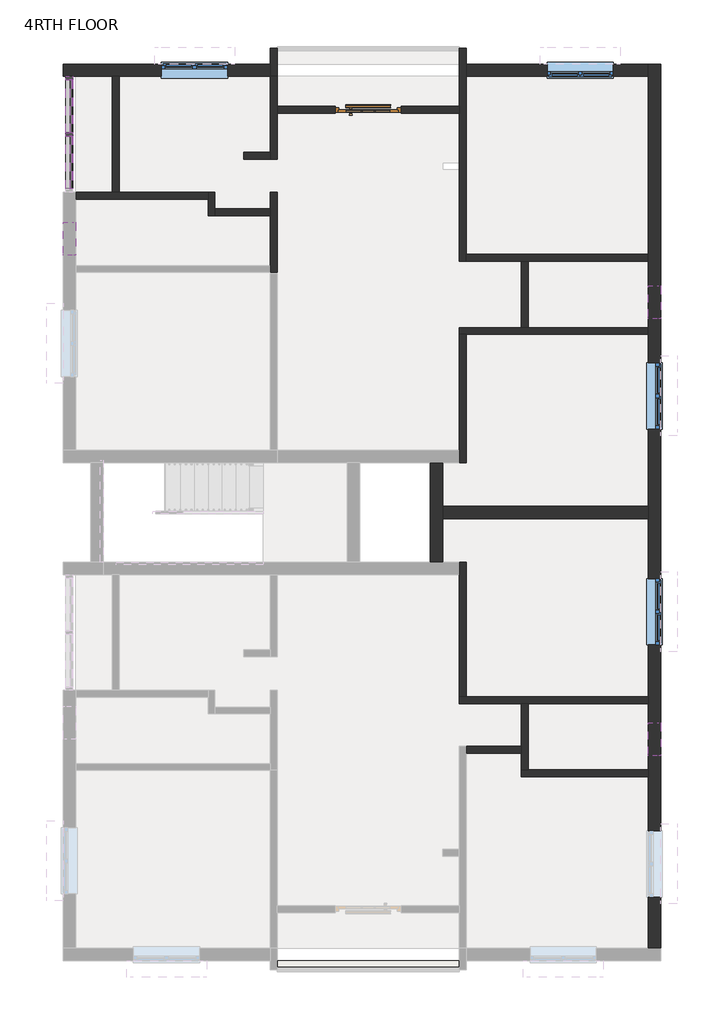
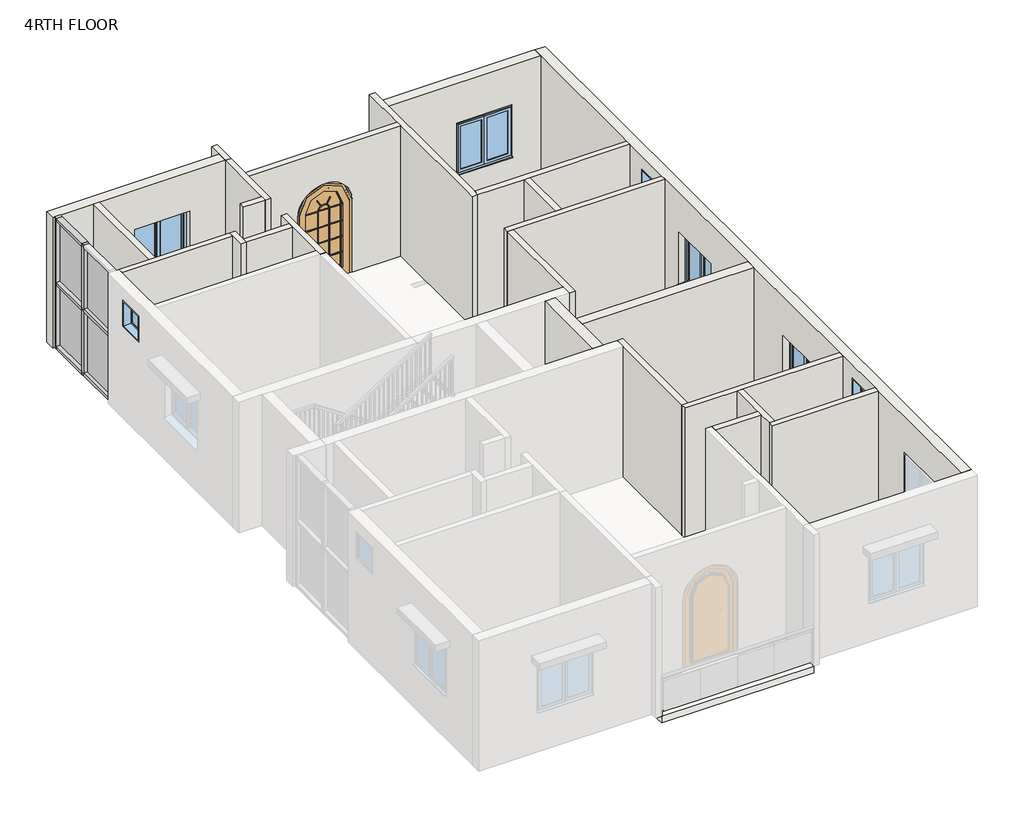
# One storey, part 2 of 4: 24 walls, 9 members, 7 windows, 4 plates, 1 door, 1 slab.
"""IFC4 building model written with IfcOpenShell, lengths in millimetres."""

from ifc_helpers import new_model, si_unit, point, frame, frame_2d, origin, place, context, project, spatial, polyline, circle_curve, trimmed, segment, composite_curve, outline, extrude, faceted_brep, transform, mapped, element, save
from components import door_arched_single_french_glass_wood_exterior_4_x_7_french_5c4dec95, member_801a2072, member_82905deb, member_88aa5c81, member_4491d118, system_panel_glazed_a8655be6, window_80340324, w2_windows_4_x_4_9dec5fc7

model = new_model("IFC4")

# Units and contexts
model_context = context("Model", 3, world=origin())
ifc_project = project(units=[si_unit("LENGTHUNIT", "METRE", prefix="MILLI")], contexts=[model_context])

# Site, building, storey
site = spatial("IfcSite", under=ifc_project)
building = spatial("IfcBuilding", under=site)
storey = spatial("IfcBuildingStorey", under=building, Name="4RTH FLOOR", Elevation=15240.0)

# Door
placement = place(None, origin())
door_arched_single_french_glass_wood_exterior_4_x_7_french_shape = door_arched_single_french_glass_wood_exterior_4_x_7_french_5c4dec95(model_context)
element("IfcDoor", 1, ObjectType="Door_Arched_Single_French_Glass_Wood_Exterior : 4' x 7' french door", at=placement, inside=storey, context=model_context, shape_type="MappedRepresentation", body=[
    mapped(door_arched_single_french_glass_wood_exterior_4_x_7_french_shape, transform((-817.6012202, 12433.0309003, 15240.0), x_axis=(1.0, 0.0, 0.0), y_axis=(0.0, 1.0, 0.0), z_axis=(0.0, 0.0, 1.0))),
])

# Members
member_shape = member_801a2072(model_context)
element("IfcMember", 2, ObjectType="Rectangular Mullion : 2.5\" x 5\" rectangular", at=placement, inside=storey, context=model_context, shape_type="MappedRepresentation", body=[
    mapped(member_shape, transform((-6318.2887202, 12007.5809003, 18288.0), x_axis=(0.0, 0.0, 1.0), y_axis=(-1.0, 0.0, 0.0), z_axis=(0.0, -1.0, 0.0))),
])
element("IfcMember", 3, ObjectType="Rectangular Mullion : 2.5\" x 5\" rectangular", at=placement, inside=storey, context=model_context, shape_type="MappedRepresentation", body=[
    mapped(member_shape, transform((-6318.2887202, 12979.1309003, 15240.0), x_axis=(0.0, 0.0, -1.0), y_axis=(-1.0, 0.0, 0.0), z_axis=(0.0, 1.0, 0.0))),
])
element("IfcMember", 4, ObjectType="Rectangular Mullion : 2.5\" x 5\" rectangular", at=placement, inside=storey, context=model_context, shape_type="MappedRepresentation", body=[
    mapped(member_shape, transform((-6318.2887202, 11944.0809003, 15240.0), x_axis=(0.0, 0.0, -1.0), y_axis=(-1.0, 0.0, 0.0), z_axis=(0.0, 1.0, 0.0))),
])
member_2_shape = member_82905deb(model_context)
element("IfcMember", 5, ObjectType="Rectangular Mullion : 2.5\" x 5\" rectangular", at=placement, inside=storey, context=model_context, shape_type="MappedRepresentation", body=[
    mapped(member_2_shape, transform((-6318.2887202, 11975.8309003, 15240.0), x_axis=(0.0, -1.0, 0.0), y_axis=(-1.0, 0.0, 0.0), z_axis=(0.0, 0.0, -1.0))),
])
member_3_shape = member_88aa5c81(model_context)
element("IfcMember", 6, ObjectType="Rectangular Mullion : 2.5\" x 5\" rectangular", at=placement, inside=storey, context=model_context, shape_type="MappedRepresentation", body=[
    mapped(member_3_shape, transform((-6318.2887202, 12007.5809003, 16764.0), x_axis=(0.0, 0.0, 1.0), y_axis=(-1.0, 0.0, 0.0), z_axis=(0.0, -1.0, 0.0))),
])
element("IfcMember", 7, ObjectType="Rectangular Mullion : 2.5\" x 5\" rectangular", at=placement, inside=storey, context=model_context, shape_type="MappedRepresentation", body=[
    mapped(member_3_shape, transform((-6318.2887202, 10972.5309003, 16764.0), x_axis=(0.0, 0.0, 1.0), y_axis=(-1.0, 0.0, 0.0), z_axis=(0.0, -1.0, 0.0))),
])
element("IfcMember", 8, ObjectType="Rectangular Mullion : 2.5\" x 5\" rectangular", at=placement, inside=storey, context=model_context, shape_type="MappedRepresentation", body=[
    mapped(member_2_shape, transform((-6318.2887202, 11975.8309003, 16764.0), x_axis=(0.0, -1.0, 0.0), y_axis=(-1.0, 0.0, 0.0), z_axis=(0.0, 0.0, -1.0))),
])
member_4_shape = member_4491d118(model_context)
element("IfcMember", 9, ObjectType="Rectangular Mullion : 2.5\" x 5\" rectangular", at=placement, inside=storey, context=model_context, shape_type="MappedRepresentation", body=[
    mapped(member_4_shape, transform((-6318.2887202, 13042.6309003, 18288.0), x_axis=(0.0, 1.0, 0.0), y_axis=(-1.0, 0.0, 0.0), z_axis=(0.0, 0.0, 1.0))),
])
element("IfcMember", 10, ObjectType="Rectangular Mullion : 2.5\" x 5\" rectangular", at=placement, inside=storey, context=model_context, shape_type="MappedRepresentation", body=[
    mapped(member_4_shape, transform((-6318.2887202, 13042.6309003, 16764.0), x_axis=(0.0, 1.0, 0.0), y_axis=(-1.0, 0.0, 0.0), z_axis=(0.0, 0.0, 1.0))),
])

# Plates
system_panel_glazed_shape = system_panel_glazed_a8655be6(model_context)
element("IfcPlate", 11, ObjectType="System Panel : Glazed", at=placement, inside=storey, context=model_context, shape_type="MappedRepresentation", body=[
    mapped(system_panel_glazed_shape, transform((-6318.2887202, 12493.3559003, 15303.5), x_axis=(0.0, -1.0, 0.0), y_axis=(1.0, 0.0, 0.0), z_axis=(0.0, 0.0, 1.0))),
])
element("IfcPlate", 12, ObjectType="System Panel : Glazed", at=placement, inside=storey, context=model_context, shape_type="MappedRepresentation", body=[
    mapped(system_panel_glazed_shape, transform((-6318.2887202, 11458.3059003, 15303.5), x_axis=(0.0, -1.0, 0.0), y_axis=(1.0, 0.0, 0.0), z_axis=(0.0, 0.0, 1.0))),
])
element("IfcPlate", 13, ObjectType="System Panel : Glazed", at=placement, inside=storey, context=model_context, shape_type="MappedRepresentation", body=[
    mapped(system_panel_glazed_shape, transform((-6318.2887202, 12493.3559003, 16795.75), x_axis=(0.0, -1.0, 0.0), y_axis=(1.0, 0.0, 0.0), z_axis=(0.0, 0.0, 1.0))),
])
element("IfcPlate", 14, ObjectType="System Panel : Glazed", at=placement, inside=storey, context=model_context, shape_type="MappedRepresentation", body=[
    mapped(system_panel_glazed_shape, transform((-6318.2887202, 11458.3059003, 16795.75), x_axis=(0.0, -1.0, 0.0), y_axis=(1.0, 0.0, 0.0), z_axis=(0.0, 0.0, 1.0))),
])

# Slab
element("IfcSlab", 15, ObjectType="bathroom tiles", at=placement, inside=storey, context=model_context, shape_type="SweptSolid", body=[
    extrude(outline(polyline([(858.7987798, -3238.7690997), (858.7987798, -3403.8690997), (-2494.0012202, -3403.8690997), (-2494.0012202, -3238.7690997), (858.7987798, -3238.7690997)])), frame((0.0, 0.0, 15087.6), z_axis=(0.0, 0.0, 1.0), x_axis=(1.0, 0.0, 0.0)), (0.0, 0.0, 1.0), 152.4),
])

# Walls
element("IfcWall", 16, ObjectType="OUTER WALL 9\"", at=placement, inside=storey, context=model_context, shape_type="Brep", body=[
    faceted_brep([(4567.1987798, -3010.1690997, 15240.0), (4567.1987798, 13271.2309003, 15240.0), (4567.1987798, 13271.2309003, 18288.0), (4567.1987798, -3010.1690997, 18288.0), (4567.1987798, -844.8190997, 16240.0), (4567.1987798, -2064.0190997, 16240.0), (4567.1987798, -2064.0190997, 17459.2), (4567.1987798, -844.8190997, 17459.2), (4567.1987798, 2577.8309003, 16154.4), (4567.1987798, 2577.8309003, 17373.6), (4567.1987798, 3797.0309003, 17373.6), (4567.1987798, 3797.0309003, 16154.4), (4567.1987798, 6552.9309003, 16154.4), (4567.1987798, 6552.9309003, 17373.6), (4567.1987798, 7772.1309003, 17373.6), (4567.1987798, 7772.1309003, 16154.4), (4567.1987798, 539.4809003, 17983.2), (4567.1987798, 1149.0809003, 17983.2), (4567.1987798, 1149.0809003, 17373.6), (4567.1987798, 539.4809003, 17373.6), (4567.1987798, 8584.9309003, 17983.2), (4567.1987798, 9194.5309003, 17983.2), (4567.1987798, 9194.5309003, 17373.6), (4567.1987798, 8584.9309003, 17373.6), (4338.5987798, -3010.1690997, 15240.0), (4338.5987798, -3010.1690997, 18288.0), (4338.5987798, 152.1309003, 18288.0), (4338.5987798, 279.1309003, 18288.0), (4338.5987798, 1498.3309003, 18288.0), (4338.5987798, 1625.3309003, 18288.0), (4338.5987798, 4901.9309003, 18288.0), (4338.5987798, 5130.5309003, 18288.0), (4338.5987798, 8292.8309003, 18288.0), (4338.5987798, 8419.8309003, 18288.0), (4338.5987798, 9639.0309003, 18288.0), (4338.5987798, 9766.0309003, 18288.0), (4338.5987798, 13042.6309003, 18288.0), (4338.5987798, 13271.2309003, 18288.0), (4338.5987798, 13271.2309003, 15240.0), (4338.5987798, 13042.6309003, 15240.0), (4338.5987798, 9766.0309003, 15240.0), (4338.5987798, 9639.0309003, 15240.0), (4338.5987798, 8419.8309003, 15240.0), (4338.5987798, 8292.8309003, 15240.0), (4338.5987798, 5130.5309003, 15240.0), (4338.5987798, 4901.9309003, 15240.0), (4338.5987798, 1625.3309003, 15240.0), (4338.5987798, 1498.3309003, 15240.0), (4338.5987798, 279.1309003, 15240.0), (4338.5987798, 152.1309003, 15240.0), (4338.5987798, -844.8190997, 16240.0), (4338.5987798, -844.8190997, 17459.2), (4338.5987798, -2064.0190997, 17459.2), (4338.5987798, -2064.0190997, 16240.0), (4338.5987798, 2577.8309003, 16154.4), (4338.5987798, 3797.0309003, 16154.4), (4338.5987798, 3797.0309003, 17373.6), (4338.5987798, 2577.8309003, 17373.6), (4338.5987798, 6552.9309003, 16154.4), (4338.5987798, 7772.1309003, 16154.4), (4338.5987798, 7772.1309003, 17373.6), (4338.5987798, 6552.9309003, 17373.6), (4338.5987798, 539.4809003, 17983.2), (4338.5987798, 539.4809003, 17373.6), (4338.5987798, 1149.0809003, 17373.6), (4338.5987798, 1149.0809003, 17983.2), (4338.5987798, 8584.9309003, 17983.2), (4338.5987798, 8584.9309003, 17373.6), (4338.5987798, 9194.5309003, 17373.6), (4338.5987798, 9194.5309003, 17983.2)], [[[0, 1, 2, 3], [4, 5, 6, 7], [8, 9, 10, 11], [12, 13, 14, 15], [16, 17, 18, 19], [20, 21, 22, 23]], [[24, 25, 26, 27, 28, 29, 30, 31, 32, 33, 34, 35, 36, 37, 38, 39, 40, 41, 42, 43, 44, 45, 46, 47, 48, 49], [50, 51, 52, 53], [54, 55, 56, 57], [58, 59, 60, 61], [62, 63, 64, 65], [66, 67, 68, 69]], [[1, 0, 24, 49, 48, 47, 46, 45, 44, 43, 42, 41, 40, 39, 38]], [[3, 2, 37, 36, 35, 34, 33, 32, 31, 30, 29, 28, 27, 26, 25]], [[0, 3, 25, 24]], [[2, 1, 38, 37]], [[51, 50, 4, 7]], [[52, 51, 7, 6]], [[53, 52, 6, 5]], [[50, 53, 5, 4]], [[9, 8, 54, 57]], [[10, 9, 57, 56]], [[11, 10, 56, 55]], [[8, 11, 55, 54]], [[13, 12, 58, 61]], [[14, 13, 61, 60]], [[15, 14, 60, 59]], [[12, 15, 59, 58]], [[63, 62, 16, 19]], [[64, 63, 19, 18]], [[65, 64, 18, 17]], [[62, 65, 17, 16]], [[67, 66, 20, 23]], [[68, 67, 23, 22]], [[69, 68, 22, 21]], [[66, 69, 21, 20]]]),
])
element("IfcWall", 17, ObjectType="OUTER WALL 9\"", at=placement, inside=storey, context=model_context, shape_type="SweptSolid", body=[
    extrude(outline(polyline([(15240.0, 4338.5987798), (18288.0, 4338.5987798), (18288.0, 985.7987798), (15240.0, 985.7987798), (15240.0, 4338.5987798)]), holes=[polyline([(16154.4, 2479.7847416), (17373.6, 2479.7847416), (17373.6, 3698.9847416), (16154.4, 3698.9847416), (16154.4, 2479.7847416)])]), frame((0.0, 13042.6309003, 0.0), z_axis=(0.0, 1.0, 0.0), x_axis=(0.0, 0.0, 1.0)), (0.0, 0.0, 1.0), 228.6),
])
element("IfcWall", 18, ObjectType="OUTER WALL 9\"", at=placement, inside=storey, context=model_context, shape_type="Brep", body=[
    faceted_brep([(-2621.0012202, 13271.2309003, 15240.0), (-6432.5887202, 13271.2309003, 15240.0), (-6432.5887202, 13271.2309003, 18288.0), (-2621.0012202, 13271.2309003, 18288.0), (-3402.0512202, 13271.2309003, 16154.4), (-3402.0512202, 13271.2309003, 17373.6), (-4621.2512202, 13271.2309003, 17373.6), (-4621.2512202, 13271.2309003, 16154.4), (-2621.0012202, 13042.6309003, 15240.0), (-2621.0012202, 13042.6309003, 18288.0), (-5402.3012202, 13042.6309003, 18288.0), (-5529.3012202, 13042.6309003, 18288.0), (-6432.5887202, 13042.6309003, 18288.0), (-6432.5887202, 13042.6309003, 15240.0), (-5529.3012202, 13042.6309003, 15240.0), (-5402.3012202, 13042.6309003, 15240.0), (-3402.0512202, 13042.6309003, 16154.4), (-4621.2512202, 13042.6309003, 16154.4), (-4621.2512202, 13042.6309003, 17373.6), (-3402.0512202, 13042.6309003, 17373.6)], [[[0, 1, 2, 3], [4, 5, 6, 7]], [[8, 9, 10, 11, 12, 13, 14, 15], [16, 17, 18, 19]], [[1, 0, 8, 15, 14, 13]], [[3, 2, 12, 11, 10, 9]], [[2, 1, 13, 12]], [[5, 4, 16, 19]], [[6, 5, 19, 18]], [[7, 6, 18, 17]], [[4, 7, 17, 16]], [[0, 3, 9, 8]]]),
])
element("IfcWall", 19, ObjectType="OUTER WALL 9\"", at=placement, inside=storey, context=model_context, shape_type="Brep", body=[
    faceted_brep([(553.9987798, 4101.8309003, 15240.0), (553.9987798, 4901.9309003, 15240.0), (553.9987798, 5130.5309003, 15240.0), (553.9987798, 5930.6309003, 15240.0), (553.9987798, 5930.6309003, 18288.0), (553.9987798, 5130.5309003, 18288.0), (553.9987798, 4901.9309003, 18288.0), (553.9987798, 4101.8309003, 18288.0), (325.3987798, 4101.8309003, 15240.0), (325.3987798, 4101.8309003, 18288.0), (325.3987798, 5930.6309003, 18288.0), (325.3987798, 5930.6309003, 15240.0)], [[[0, 1, 2, 3, 4, 5, 6, 7]], [[8, 9, 10, 11]], [[3, 2, 1, 0, 8, 11]], [[7, 6, 5, 4, 10, 9]], [[0, 7, 9, 8]], [[4, 3, 11, 10]]]),
])
element("IfcWall", 20, ObjectType="OUTER WALL 9\"", at=placement, inside=storey, context=model_context, shape_type="SweptSolid", body=[
    extrude(outline(polyline([(4338.5987798, 4901.9309003), (553.9987798, 4901.9309003), (553.9987798, 5130.5309003), (4338.5987798, 5130.5309003), (4338.5987798, 4901.9309003)])), frame((0.0, 0.0, 15240.0), z_axis=(0.0, 0.0, 1.0), x_axis=(1.0, 0.0, 0.0)), (0.0, 0.0, 1.0), 3048.0),
])
element("IfcWall", 21, ObjectType="inner wall 5\"", at=placement, inside=storey, context=model_context, shape_type="SweptSolid", body=[
    extrude(outline(polyline([(-5529.3012202, 10909.0309003), (-5529.3012202, 13042.6309003), (-5402.3012202, 13042.6309003), (-5402.3012202, 10909.0309003), (-5529.3012202, 10909.0309003)])), frame((0.0, 0.0, 15240.0), z_axis=(0.0, 0.0, 1.0), x_axis=(1.0, 0.0, 0.0)), (0.0, 0.0, 1.0), 3048.0),
])
element("IfcWall", 22, ObjectType="inner wall 5\"", at=placement, inside=storey, context=model_context, shape_type="Brep", body=[
    faceted_brep([(-2621.0012202, 13042.6309003, 15240.0), (-2621.0012202, 11645.6309003, 15240.0), (-2621.0012202, 11518.6309003, 15240.0), (-2621.0012202, 11518.6309003, 18288.0), (-2621.0012202, 11645.6309003, 18288.0), (-2621.0012202, 13042.6309003, 18288.0), (-2494.0012202, 13042.6309003, 15240.0), (-2494.0012202, 13042.6309003, 18288.0), (-2494.0012202, 12496.5309003, 18288.0), (-2494.0012202, 12369.5309003, 18288.0), (-2494.0012202, 11518.6309003, 18288.0), (-2494.0012202, 11518.6309003, 15240.0), (-2494.0012202, 12369.5309003, 15240.0), (-2494.0012202, 12496.5309003, 15240.0)], [[[0, 1, 2, 3, 4, 5]], [[6, 7, 8, 9, 10, 11, 12, 13]], [[2, 1, 0, 6, 13, 12, 11]], [[5, 4, 3, 10, 9, 8, 7]], [[3, 2, 11, 10]], [[0, 5, 7, 6]]]),
])
element("IfcWall", 23, ObjectType="inner wall 5\"", at=placement, inside=storey, context=model_context, shape_type="SweptSolid", body=[
    extrude(outline(polyline([(-3103.6012202, 11645.6309003), (-2621.0012202, 11645.6309003), (-2621.0012202, 11518.6309003), (-3103.6012202, 11518.6309003), (-3103.6012202, 11645.6309003)])), frame((0.0, 0.0, 15240.0), z_axis=(0.0, 0.0, 1.0), x_axis=(1.0, 0.0, 0.0)), (0.0, 0.0, 1.0), 3048.0),
])
element("IfcWall", 24, ObjectType="inner wall 5\"", at=placement, inside=storey, context=model_context, shape_type="Brep", body=[
    faceted_brep([(-6202.4012202, 10782.0309003, 15240.0), (-3764.0012202, 10782.0309003, 15240.0), (-3764.0012202, 10782.0309003, 18288.0), (-6202.4012202, 10782.0309003, 18288.0), (-6202.4012202, 10909.0309003, 15240.0), (-6202.4012202, 10909.0309003, 18288.0), (-5529.3012202, 10909.0309003, 18288.0), (-5402.3012202, 10909.0309003, 18288.0), (-3764.0012202, 10909.0309003, 18288.0), (-3764.0012202, 10909.0309003, 15240.0), (-5402.3012202, 10909.0309003, 15240.0), (-5529.3012202, 10909.0309003, 15240.0)], [[[0, 1, 2, 3]], [[4, 5, 6, 7, 8, 9, 10, 11]], [[1, 0, 4, 11, 10, 9]], [[3, 2, 8, 7, 6, 5]], [[0, 3, 5, 4]], [[2, 1, 9, 8]]]),
])
element("IfcWall", 25, ObjectType="inner wall 5\"", at=placement, inside=storey, context=model_context, shape_type="Brep", body=[
    faceted_brep([(-3764.0012202, 10909.0309003, 15240.0), (-3764.0012202, 10782.0309003, 15240.0), (-3764.0012202, 10477.2309003, 15240.0), (-3764.0012202, 10477.2309003, 18288.0), (-3764.0012202, 10782.0309003, 18288.0), (-3764.0012202, 10909.0309003, 18288.0), (-3637.0012202, 10909.0309003, 15240.0), (-3637.0012202, 10909.0309003, 18288.0), (-3637.0012202, 10604.2309003, 18288.0), (-3637.0012202, 10477.2309003, 18288.0), (-3637.0012202, 10477.2309003, 15240.0), (-3637.0012202, 10604.2309003, 15240.0)], [[[0, 1, 2, 3, 4, 5]], [[6, 7, 8, 9, 10, 11]], [[2, 1, 0, 6, 11, 10]], [[5, 4, 3, 9, 8, 7]], [[0, 5, 7, 6]], [[3, 2, 10, 9]]]),
])
element("IfcWall", 26, ObjectType="inner wall 5\"", at=placement, inside=storey, context=model_context, shape_type="SweptSolid", body=[
    extrude(outline(polyline([(-2621.0012202, 10477.2309003), (-3637.0012202, 10477.2309003), (-3637.0012202, 10604.2309003), (-2621.0012202, 10604.2309003), (-2621.0012202, 10477.2309003)])), frame((0.0, 0.0, 15240.0), z_axis=(0.0, 0.0, 1.0), x_axis=(1.0, 0.0, 0.0)), (0.0, 0.0, 1.0), 3048.0),
])
element("IfcWall", 27, ObjectType="inner wall 5\"", at=placement, inside=storey, context=model_context, shape_type="Brep", body=[
    faceted_brep([(-2621.0012202, 10909.0309003, 15240.0), (-2621.0012202, 10604.2309003, 15240.0), (-2621.0012202, 10477.2309003, 15240.0), (-2621.0012202, 9562.8309003, 15240.0), (-2621.0012202, 9435.8309003, 15240.0), (-2621.0012202, 9435.8309003, 18288.0), (-2621.0012202, 9562.8309003, 18288.0), (-2621.0012202, 10477.2309003, 18288.0), (-2621.0012202, 10604.2309003, 18288.0), (-2621.0012202, 10909.0309003, 18288.0), (-2494.0012202, 10909.0309003, 15240.0), (-2494.0012202, 10909.0309003, 18288.0), (-2494.0012202, 9435.8309003, 18288.0), (-2494.0012202, 9435.8309003, 15240.0)], [[[0, 1, 2, 3, 4, 5, 6, 7, 8, 9]], [[10, 11, 12, 13]], [[4, 3, 2, 1, 0, 10, 13]], [[9, 8, 7, 6, 5, 12, 11]], [[0, 9, 11, 10]], [[5, 4, 13, 12]]]),
])
element("IfcWall", 28, ObjectType="inner wall 5\"", at=placement, inside=storey, context=model_context, shape_type="SweptSolid", body=[
    extrude(outline(polyline([(2001.7987798, 583.9309003), (985.7987798, 583.9309003), (985.7987798, 710.9309003), (2001.7987798, 710.9309003), (2001.7987798, 583.9309003)])), frame((0.0, 0.0, 15240.0), z_axis=(0.0, 0.0, 1.0), x_axis=(1.0, 0.0, 0.0)), (0.0, 0.0, 1.0), 3048.0),
])
element("IfcWall", 29, ObjectType="inner wall 5\"", at=placement, inside=storey, context=model_context, shape_type="Brep", body=[
    faceted_brep([(4338.5987798, 1625.3309003, 15240.0), (985.7987798, 1625.3309003, 15240.0), (858.7987798, 1625.3309003, 15240.0), (858.7987798, 1625.3309003, 18288.0), (985.7987798, 1625.3309003, 18288.0), (4338.5987798, 1625.3309003, 18288.0), (4338.5987798, 1498.3309003, 15240.0), (4338.5987798, 1498.3309003, 18288.0), (2128.7987798, 1498.3309003, 18288.0), (2001.7987798, 1498.3309003, 18288.0), (858.7987798, 1498.3309003, 18288.0), (858.7987798, 1498.3309003, 15240.0), (2001.7987798, 1498.3309003, 15240.0), (2128.7987798, 1498.3309003, 15240.0)], [[[0, 1, 2, 3, 4, 5]], [[6, 7, 8, 9, 10, 11, 12, 13]], [[2, 1, 0, 6, 13, 12, 11]], [[5, 4, 3, 10, 9, 8, 7]], [[3, 2, 11, 10]], [[0, 5, 7, 6]]]),
])
element("IfcWall", 30, ObjectType="inner wall 5\"", at=placement, inside=storey, context=model_context, shape_type="Brep", body=[
    faceted_brep([(985.7987798, 1625.3309003, 15240.0), (985.7987798, 4101.8309003, 15240.0), (985.7987798, 4101.8309003, 18288.0), (985.7987798, 1625.3309003, 18288.0), (858.7987798, 1625.3309003, 15240.0), (858.7987798, 1625.3309003, 18288.0), (858.7987798, 3873.2309003, 18288.0), (858.7987798, 4101.8309003, 18288.0), (858.7987798, 4101.8309003, 15240.0), (858.7987798, 3873.2309003, 15240.0)], [[[0, 1, 2, 3]], [[4, 5, 6, 7, 8, 9]], [[1, 0, 4, 9, 8]], [[3, 2, 7, 6, 5]], [[0, 3, 5, 4]], [[2, 1, 8, 7]]]),
])
element("IfcWall", 31, ObjectType="inner wall 5\"", at=placement, inside=storey, context=model_context, shape_type="Brep", body=[
    faceted_brep([(4338.5987798, 279.1309003, 15240.0), (2128.7987798, 279.1309003, 15240.0), (2001.7987798, 279.1309003, 15240.0), (2001.7987798, 279.1309003, 18288.0), (2128.7987798, 279.1309003, 18288.0), (4338.5987798, 279.1309003, 18288.0), (4338.5987798, 152.1309003, 15240.0), (4338.5987798, 152.1309003, 18288.0), (2001.7987798, 152.1309003, 18288.0), (2001.7987798, 152.1309003, 15240.0)], [[[0, 1, 2, 3, 4, 5]], [[6, 7, 8, 9]], [[2, 1, 0, 6, 9]], [[5, 4, 3, 8, 7]], [[0, 5, 7, 6]], [[3, 2, 9, 8]]]),
])
element("IfcWall", 32, ObjectType="inner wall 5\"", at=placement, inside=storey, context=model_context, shape_type="Brep", body=[
    faceted_brep([(2128.7987798, 279.1309003, 15240.0), (2128.7987798, 1498.3309003, 15240.0), (2128.7987798, 1498.3309003, 18288.0), (2128.7987798, 279.1309003, 18288.0), (2001.7987798, 279.1309003, 15240.0), (2001.7987798, 279.1309003, 18288.0), (2001.7987798, 583.9309003, 18288.0), (2001.7987798, 710.9309003, 18288.0), (2001.7987798, 1498.3309003, 18288.0), (2001.7987798, 1498.3309003, 15240.0), (2001.7987798, 710.9309003, 15240.0), (2001.7987798, 583.9309003, 15240.0)], [[[0, 1, 2, 3]], [[4, 5, 6, 7, 8, 9, 10, 11]], [[1, 0, 4, 11, 10, 9]], [[3, 2, 8, 7, 6, 5]], [[0, 3, 5, 4]], [[2, 1, 9, 8]]]),
])
element("IfcWall", 33, ObjectType="inner wall 5\"", at=placement, inside=storey, context=model_context, shape_type="SweptSolid", body=[
    extrude(outline(composite_curve([segment(polyline([(16918.6, -208.0012202), (15240.0, -208.0012202), (15240.0, 858.7987798), (18288.0, 858.7987798), (18288.0, -2494.0012202), (15240.0, -2494.0012202), (15240.0, -1427.2012202), (16918.6, -1427.2012202)]), True, "CONTINUOUS"), segment(trimmed(circle_curve(frame_2d((16918.6, -817.6012202)), 609.6), [point((16918.6, -1427.2012202))], [point((16918.6, -208.0012202))], True, "CARTESIAN"), True, "CONTINUOUS")], self_intersect=False)), frame((0.0, 12369.5309003, 0.0), z_axis=(0.0, 1.0, 0.0), x_axis=(0.0, 0.0, 1.0)), (0.0, 0.0, 1.0), 127.0),
])
element("IfcWall", 34, ObjectType="inner wall 5\"", at=placement, inside=storey, context=model_context, shape_type="Brep", body=[
    faceted_brep([(858.7987798, 13563.3309003, 15240.0), (858.7987798, 12496.5309003, 15240.0), (858.7987798, 12369.5309003, 15240.0), (858.7987798, 9639.0309003, 15240.0), (858.7987798, 9639.0309003, 18288.0), (858.7987798, 12369.5309003, 18288.0), (858.7987798, 12496.5309003, 18288.0), (858.7987798, 13563.3309003, 18288.0), (985.7987798, 13563.3309003, 15240.0), (985.7987798, 13563.3309003, 18288.0), (985.7987798, 13271.2309003, 18288.0), (985.7987798, 13042.6309003, 18288.0), (985.7987798, 9766.0309003, 18288.0), (985.7987798, 9639.0309003, 18288.0), (985.7987798, 9639.0309003, 15240.0), (985.7987798, 9766.0309003, 15240.0), (985.7987798, 13042.6309003, 15240.0), (985.7987798, 13271.2309003, 15240.0)], [[[0, 1, 2, 3, 4, 5, 6, 7]], [[8, 9, 10, 11, 12, 13, 14, 15, 16, 17]], [[3, 2, 1, 0, 8, 17, 16, 15, 14]], [[7, 6, 5, 4, 13, 12, 11, 10, 9]], [[0, 7, 9, 8]], [[4, 3, 14, 13]]]),
])
element("IfcWall", 35, ObjectType="inner wall 5\"", at=placement, inside=storey, context=model_context, shape_type="Brep", body=[
    faceted_brep([(4338.5987798, 9766.0309003, 15240.0), (985.7987798, 9766.0309003, 15240.0), (985.7987798, 9766.0309003, 18288.0), (4338.5987798, 9766.0309003, 18288.0), (4338.5987798, 9639.0309003, 15240.0), (4338.5987798, 9639.0309003, 18288.0), (2128.7987798, 9639.0309003, 18288.0), (2001.7987798, 9639.0309003, 18288.0), (985.7987798, 9639.0309003, 18288.0), (985.7987798, 9639.0309003, 15240.0), (2001.7987798, 9639.0309003, 15240.0), (2128.7987798, 9639.0309003, 15240.0)], [[[0, 1, 2, 3]], [[4, 5, 6, 7, 8, 9, 10, 11]], [[1, 0, 4, 11, 10, 9]], [[3, 2, 8, 7, 6, 5]], [[0, 3, 5, 4]], [[2, 1, 9, 8]]]),
])
element("IfcWall", 36, ObjectType="inner wall 5\"", at=placement, inside=storey, context=model_context, shape_type="Brep", body=[
    faceted_brep([(4338.5987798, 8419.8309003, 15240.0), (2128.7987798, 8419.8309003, 15240.0), (2001.7987798, 8419.8309003, 15240.0), (858.7987798, 8419.8309003, 15240.0), (858.7987798, 8419.8309003, 18288.0), (2001.7987798, 8419.8309003, 18288.0), (2128.7987798, 8419.8309003, 18288.0), (4338.5987798, 8419.8309003, 18288.0), (4338.5987798, 8292.8309003, 15240.0), (4338.5987798, 8292.8309003, 18288.0), (985.7987798, 8292.8309003, 18288.0), (858.7987798, 8292.8309003, 18288.0), (858.7987798, 8292.8309003, 15240.0), (985.7987798, 8292.8309003, 15240.0)], [[[0, 1, 2, 3, 4, 5, 6, 7]], [[8, 9, 10, 11, 12, 13]], [[3, 2, 1, 0, 8, 13, 12]], [[7, 6, 5, 4, 11, 10, 9]], [[0, 7, 9, 8]], [[4, 3, 12, 11]]]),
])
element("IfcWall", 37, ObjectType="inner wall 5\"", at=placement, inside=storey, context=model_context, shape_type="SweptSolid", body=[
    extrude(outline(polyline([(2128.7987798, 9639.0309003), (2128.7987798, 8419.8309003), (2001.7987798, 8419.8309003), (2001.7987798, 9639.0309003), (2128.7987798, 9639.0309003)])), frame((0.0, 0.0, 15240.0), z_axis=(0.0, 0.0, 1.0), x_axis=(1.0, 0.0, 0.0)), (0.0, 0.0, 1.0), 3048.0),
])
element("IfcWall", 38, ObjectType="inner wall 5\"", at=placement, inside=storey, context=model_context, shape_type="Brep", body=[
    faceted_brep([(858.7987798, 8292.8309003, 15240.0), (858.7987798, 6159.2309003, 15240.0), (858.7987798, 5930.6309003, 15240.0), (858.7987798, 5930.6309003, 18288.0), (858.7987798, 6159.2309003, 18288.0), (858.7987798, 8292.8309003, 18288.0), (985.7987798, 8292.8309003, 15240.0), (985.7987798, 8292.8309003, 18288.0), (985.7987798, 5930.6309003, 18288.0), (985.7987798, 5930.6309003, 15240.0)], [[[0, 1, 2, 3, 4, 5]], [[6, 7, 8, 9]], [[2, 1, 0, 6, 9]], [[5, 4, 3, 8, 7]], [[0, 5, 7, 6]], [[3, 2, 9, 8]]]),
])
element("IfcWall", 39, ObjectType="inner wall 5\"", at=placement, inside=storey, context=model_context, shape_type="Brep", body=[
    faceted_brep([(-2494.0012202, 13042.6309003, 15240.0), (-2494.0012202, 13563.3309003, 15240.0), (-2494.0012202, 13563.3309003, 18288.0), (-2494.0012202, 13042.6309003, 18288.0), (-2621.0012202, 13042.6309003, 15240.0), (-2621.0012202, 13042.6309003, 18288.0), (-2621.0012202, 13271.2309003, 18288.0), (-2621.0012202, 13563.3309003, 18288.0), (-2621.0012202, 13563.3309003, 15240.0), (-2621.0012202, 13271.2309003, 15240.0)], [[[0, 1, 2, 3]], [[4, 5, 6, 7, 8, 9]], [[1, 0, 4, 9, 8]], [[2, 1, 8, 7]], [[3, 2, 7, 6, 5]], [[0, 3, 5, 4]]]),
])

# Windows
window_shape = window_80340324(model_context)
element("IfcWindow", 40, ObjectType="Fixed : 24\" x 24\"", at=placement, inside=storey, context=model_context, shape_type="MappedRepresentation", body=[
    mapped(window_shape, transform((4452.8987798, 8851.6309003, 16459.2), x_axis=(0.0, -1.0, 0.0), y_axis=(1.0, 0.0, 0.0), z_axis=(0.0, 0.0, 1.0))),
])
element("IfcWindow", 41, ObjectType="Fixed : 24\" x 24\"", at=placement, inside=storey, context=model_context, shape_type="MappedRepresentation", body=[
    mapped(window_shape, transform((4452.8987798, 806.1809003, 16459.2), x_axis=(0.0, -1.0, 0.0), y_axis=(1.0, 0.0, 0.0), z_axis=(0.0, 0.0, 1.0))),
])
element("IfcWindow", 42, ObjectType="Fixed : 24\" x 24\"", at=placement, inside=storey, context=model_context, shape_type="MappedRepresentation", body=[
    mapped(window_shape, transform((-6318.2887202, 10020.0309003, 16459.2), x_axis=(0.0, -1.0, 0.0), y_axis=(1.0, 0.0, 0.0), z_axis=(0.0, 0.0, 1.0))),
])
w2_windows_4_x_4_shape = w2_windows_4_x_4_9dec5fc7(model_context)
element("IfcWindow", 43, ObjectType="w2 : windows 4' x 4'", at=placement, inside=storey, context=model_context, shape_type="MappedRepresentation", body=[
    mapped(w2_windows_4_x_4_shape, transform((3089.3847416, 13156.9309003, 15154.4), x_axis=(1.0, 0.0, 0.0), y_axis=(0.0, 1.0, 0.0), z_axis=(0.0, 0.0, 1.0))),
])
element("IfcWindow", 44, ObjectType="w2 : windows 4' x 4'", at=placement, inside=storey, context=model_context, shape_type="MappedRepresentation", body=[
    mapped(w2_windows_4_x_4_shape, transform((-4011.6512202, 13156.9309003, 15154.4), x_axis=(-1.0, 0.0, 0.0), y_axis=(0.0, -1.0, 0.0), z_axis=(0.0, 0.0, 1.0))),
])
element("IfcWindow", 45, ObjectType="w2 : windows 4' x 4'", at=placement, inside=storey, context=model_context, shape_type="MappedRepresentation", body=[
    mapped(w2_windows_4_x_4_shape, transform((4452.8987798, 7162.5309003, 15154.4), x_axis=(0.0, 1.0, 0.0), y_axis=(-1.0, 0.0, 0.0), z_axis=(0.0, 0.0, 1.0))),
])
element("IfcWindow", 46, ObjectType="w2 : windows 4' x 4'", at=placement, inside=storey, context=model_context, shape_type="MappedRepresentation", body=[
    mapped(w2_windows_4_x_4_shape, transform((4452.8987798, 3187.4309003, 15154.4), x_axis=(0.0, 1.0, 0.0), y_axis=(-1.0, 0.0, 0.0), z_axis=(0.0, 0.0, 1.0))),
])

save(model, "model.ifc")

# Revit data of these elements
# Type "Door_Arched_Single_French_Glass_Wood_Exterior : 4' x 7' french door"
#   Type Mark = "17"
#   Type Comments = "External Single"
#   Operation = "SingleSwingRight"
#   Keynote = "L20"
#   Analytic Construction = "<None>"
#   Wrap Layers (Int) from Ext = 0' - 6.98819"
#   Wrap Layers (Ext) from Ext = 0' - 4.03543"
#   Thickness = 0' - 1.73228"
#   Stile Shutting = 0' - 5.90551"
#   Stile - Top Rail = 0' - 5.90551"
#   Stile - Hanging = 0' - 5.90551"
#   Stile - Bottom Rail = 0' - 6.88976"
#   Rough Width = 4' - 0"
#   Rough Height = 7' - 0"
#   O/A Frame Width = 0' - 2.51969"
#   Handle Z Distance = 3' - 5.33858"
#   Glazing Thickness = 0' - 0.94488"
#   Glazing Bar Thickness = 0' - 0.7874"
#   FrameWidth = 0' - 1.65354"
#   FrameOffset - External = 0' - 0.98425"
#   FrameDepth = 0' - 3.50394"
#   Door Panel Width = 3' - 7.94488"
#   Handle X Distance = 0' - 2.95276"
#   Height = 7' - 0"
#   Structural Tolerance = 0' - 0.25591"
#   Tolerance = 0' - 0.11811"
#   Undercut = 0' - 0.15748"
#   Width = 4' - 0"
#   Door Panel Thickness = 0' - 1.73228"
#   Door Panel Height = 6' - 9.81496"
#   Cavity Closer Width = 0' - 1.9685"
#   Cavity Closer Offset from Ext = 0' - 4.03543"
#   Cavity Closer Depth = 0' - 3.34646"
#   Vis - Ironmongery = yes
#   Vis - Cavity Closers = yes
#   Define Thermal Properties by = 1
#   Material Glass = Door - Glazing
#   Handle Style = element 430241
#   Material Door = Door - Panel
#   Material Frame = BROWN
#   Material Ironmongery = Door - Handle
#   Function = (empty or 0)
#   Wall Closure = (empty or 0)
#   Assembly Code = ""
# Type "Rectangular Mullion : 2.5\" x 5\" rectangular"
#   built-in parameter 1007304 = 0.416667 (stored number, unit not read)
#   built-in parameter 1007301 = 0.104167 (stored number, unit not read)
#   built-in parameter 1007300 = 0.104167 (stored number, unit not read)
# Type "System Panel : Glazed"
#   Construction Type Id = "GSP4R"
#   Analytic Construction = "1/8 in Pilkington single glazing"
#   Visual Light Transmittance = 0.9
#   Solar Heat Gain Coefficient = 0.86
#   Heat Transfer Coefficient (U) = 1.18115 BTU/(h·ft²·°F)
#   Define Thermal Properties by = 1
# Type "bathroom tiles"
#   Assembly Code = "B1010"
#   Function = 0
#   Layers, outside or top first: 0' - 6" "tile flooring" (function 1)
# Type "OUTER WALL 9\""
#   Assembly Code = "B2010"
#   Layers, outside or top first: 0' - 9" "ROSE COLOUR" (function 1)
# Type "inner wall 5\""
#   Assembly Code = "B2010"
#   Layers, outside or top first: 0' - 5" "ROSE COLOUR" (function 1)
# Type "Fixed : 24\" x 24\""
#   Type Mark = "3"
#   Construction Type Id = "GSP4R"
#   Assembly Code = "B2020100"
#   Analytic Construction = "1/8 in Pilkington single glazing"
#   Visual Light Transmittance = 0.9
#   Solar Heat Gain Coefficient = 0.78
#   Heat Transfer Coefficient (U) = 0.6496 BTU/(h·ft²·°F)
#   Height = 2' - 0"
#   Default Sill Height = 3' - 0"
#   Width = 2' - 0"
#   Window Inset = 0' - 0 3/4"
#   Define Thermal Properties by = 1
#   Define Thermal Properties by = 1
#   Glass Pane Material = Glass
#   Sash Material = Sash
#   Wall Closure = (empty or 0)
# Type "w2 : windows 4' x 4'"
#   Type Mark = "31"
#   Operation = "DoublePanelVertical"
#   Keynote = "16.05.01"
#   Analytic Construction = "<None>"
#   Rough Width = 4' - 0"
#   Rough Height = 4' - 0"
#   Rahmentiefe = 0' - 2.3622"
#   Rahmenhöhe unten = 0' - 3.14961"
#   Rahmehöhe oben = 0' - 3.14961"
#   Rahmenbreite = 0' - 2.3622"
#   Heat Transfer Coefficient (U) = 2.81836 BTU/(h·ft²·°F)
#   Height = 4' - 0"
#   Flügeltiefe = 0' - 2.3622"
#   Flügelbreite = 0' - 2.3622"
#   Einbautiefe (von außen) [instance default] = 0' - 5.51181"
#   Width = 4' - 0"
#   Kippflügel [instance default] = yes
#   Drehflügel im Grundriß darstellen [instance default] = no
#   Drehflügel [instance default] = yes
#   Define Thermal Properties by = 1
#   Rahmen [instance default] = none
#   Glas [instance default] = blue glass
#   Flügel [instance default] = WINDOW COLOUR WHITE
#   Fensterbank aussen [instance default] = WINDOW COLOUR WHITE
#   Fensterbank innen [instance default] = WINDOW COLOUR WHITE
#   Visual Light Transmittance = 0
#   Thermal Resistance (R) = 0
#   Solar Heat Gain Coefficient = 0
#   Wall Closure = (empty or 0)
# Element 1 (IfcDoor, "Door_Arched_Single_French_Glass_Wood_Exterior : 4' x 7' french door")
#   Phase Created = New Construction
#   Materials on its faces: "Door - Panel", "Door - Handle", "BROWN", "Door - Glazing"
# Elements 2, 3, 4, 5, 6, 7, 8, 9, 10 (IfcMember, "Rectangular Mullion : 2.5\" x 5\" rectangular")
#   Phase Created = New Construction
#   Materials on its faces: "Aluminum"
# Elements 11, 12, 13, 14 (IfcPlate, "System Panel : Glazed")
#   Phase Created = New Construction
#   Materials on its faces: "Glass"
# Element 15 (IfcSlab, "bathroom tiles")
#   Height Offset From Level = 0' - 0"
#   Phase Created = New Construction
#   Materials on its faces: "tile flooring"
# Elements 16, 17, 18, 19, 20 (IfcWall, "OUTER WALL 9\"")
#   Top Offset = 0' - 0"
#   Base Offset = 0' - 0"
#   wall height = 10' - 0"
#   Phase Created = New Construction
#   Base Constraint = 4RTH FLOOR
#   Top Constraint = 5th floor
#   Materials on its faces: "ROSE COLOUR"
# Elements 21, 22, 23, 24, 25, 26, 27, 28, 29, 30, 31, 32, 33, 34, 35, 36, 37, 38, 39 (IfcWall, "inner wall 5\"")
#   Top Offset = 0' - 0"
#   Base Offset = 0' - 0"
#   wall height = 10' - 0"
#   Phase Created = New Construction
#   Base Constraint = 4RTH FLOOR
#   Top Constraint = 5th floor
#   Materials on its faces: "ROSE COLOUR"
# Element 40 (IfcWindow, "Fixed : 24\" x 24\"")
#   Mark = "76"
#   Phase Created = New Construction
#   Materials on its faces: "Sash", "Glass"
# Element 41 (IfcWindow, "Fixed : 24\" x 24\"")
#   Mark = "78"
#   Phase Created = New Construction
#   Materials on its faces: "Sash", "Glass"
# Element 42 (IfcWindow, "Fixed : 24\" x 24\"")
#   Mark = "79"
#   Phase Created = New Construction
#   Materials on its faces: "Sash", "Glass"
# Element 43 (IfcWindow, "w2 : windows 4' x 4'")
#   Mark = "67"
#   Phase Created = New Construction
#   Materials on its faces: "WINDOW COLOUR WHITE", "blue glass"
# Element 44 (IfcWindow, "w2 : windows 4' x 4'")
#   Mark = "68"
#   Phase Created = New Construction
#   Materials on its faces: "WINDOW COLOUR WHITE", "blue glass"
# Element 45 (IfcWindow, "w2 : windows 4' x 4'")
#   Mark = "71"
#   Phase Created = New Construction
#   Materials on its faces: "WINDOW COLOUR WHITE", "blue glass"
# Element 46 (IfcWindow, "w2 : windows 4' x 4'")
#   Mark = "72"
#   Phase Created = New Construction
#   Materials on its faces: "WINDOW COLOUR WHITE", "blue glass"
# Materials
#   "Door - Glazing": colour RGB 218 227 224, transparency 0.85
#   "Door - Panel": class "Wood", colour RGB 210 159 95, transparency 0, Cost = 0
#   "BROWN": class "Generic", colour RGB 120 120 120, transparency 0, Cost = 0
#   "Door - Handle": colour RGB 0 0 0, transparency 0, Keynote = "P21"
#   "tile flooring": class "Generic", colour RGB 120 120 120, transparency 0, Cost = 0
#   "ROSE COLOUR": class "Generic", colour RGB 120 120 120, transparency 0, Cost = 0
#   "Glass": class "Glass", colour RGB 0 128 192, transparency 0.75, Description = "Soda Lime Glass", Cost = 0
#   "Sash": class "Wood", colour RGB 224 178 126, transparency 0, Cost = 0
#   "blue glass": class "System", colour RGB 0 0 255, transparency 0.75, Cost = 0
#   "WINDOW COLOUR WHITE": class "Generic", colour RGB 120 120 120, transparency 0, Cost = 0
#   "Aluminum": class "Metal", colour RGB 247 247 247, transparency 0, Description = "Aluminum 6061", Cost = 0
